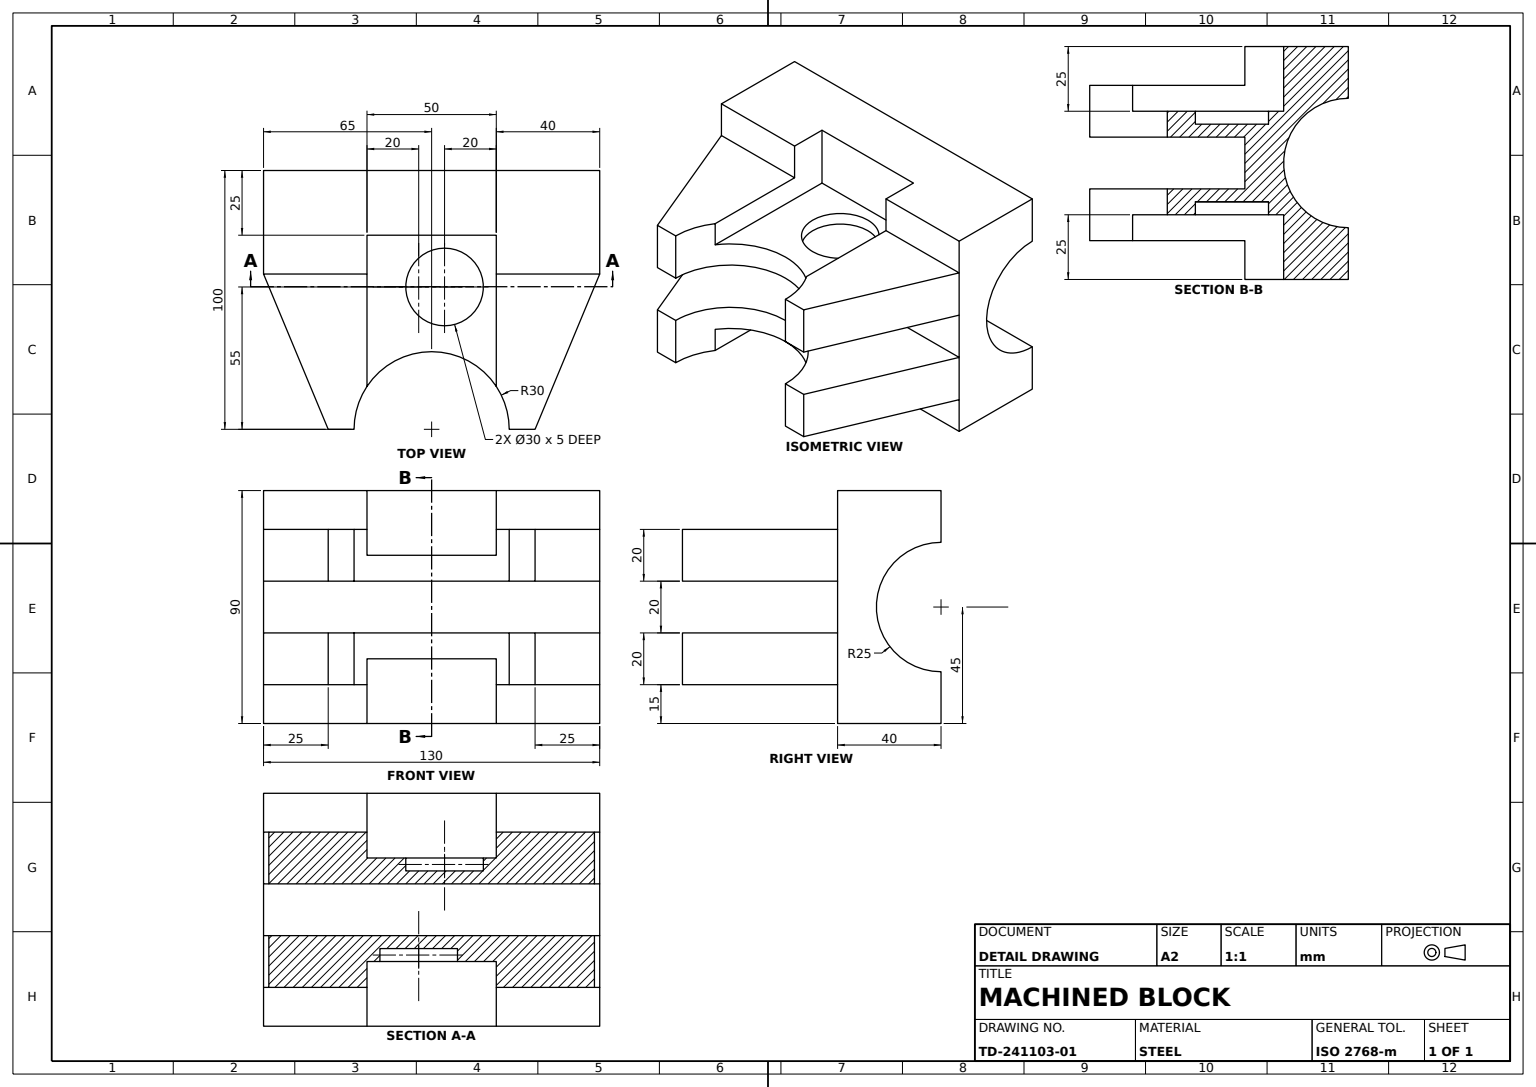
SolidWorks part; units mm, degrees
material "Plain Carbon Steel"
ref_plane "Front Plane" through (0, 0, 0) normal (0, 0, 1) x (1, 0, 0)
ref_plane "Top Plane" through (0, 0, 0) normal (0, 1, 0) x (1, 0, 0)
ref_plane "Right Plane" through (0, 0, 0) normal (1, 0, 0) x (0, 0, -1)
sketch "Base Block Sketch" plane through (0, 0, 0) normal (0, 0, 1) x (1, 0, 0)
  line L0 (0, 0) -> (130, 0)
  line L1 (130, 0) -> (130, 90)
  line L2 (130, 90) -> (0, 90)
  line L3 (0, 90) -> (0, 0)
  dimension "D1" = 130
  dimension "D2" = 90
extrude "Base Block 40" add sketch "Base Block Sketch" along normal blind 40
sketch "Side Pocket A Sketch" plane through (0, 0, 0) normal (0, -1, 0) x (1, 0, 0)
  line L0 (65, 40) -> (40, 40)
  line L1 (0, 40) -> (130, 40) construction
  line L2 (40, 40) -> (40, 25)
  line L3 (40, 25) -> (90, 25)
  line L4 (90, 25) -> (90, 40)
  line L5 (90, 40) -> (65, 40)
  line L6 (130, 40) -> (130, 0) construction
  line L7 (0, 0) -> (130, 0) construction
  dimension "D1" = 40
  dimension "D2" = 25
extrude "Side Pocket A 25" cut sketch "Side Pocket A Sketch" against normal blind 25
sketch "Side Pocket B Sketch" plane through (0, 90, 0) normal (0, 1, 0) x (1, 0, 0)
  line L0 (65, -40) -> (90, -40)
  line L1 (130, -40) -> (0, -40) construction
  line L2 (90, -40) -> (90, -25)
  line L3 (90, -25) -> (40, -25)
  line L4 (40, -25) -> (40, -40)
  line L5 (40, -40) -> (65, -40)
  line L6 (0, -40) -> (0, 0) construction
  line L7 (130, 0) -> (0, 0) construction
  dimension "D1" = 40
  dimension "D2" = 25
extrude "Side Pocket B 25" cut sketch "Side Pocket B Sketch" against normal blind 25
sketch "Upper Boss Sketch" plane through (0, 25, 0) normal (0, -1, 0) x (1, 0, 0)
  line L0 (40, 40) -> (40, 25) construction
  line L1 (90, 40) -> (40, 40) construction
  line L2 (65, 100) -> (105, 100)
  line L3 (105, 100) -> (130, 40)
  line L4 (130, 40) -> (0, 40)
  line L5 (65, 100) -> (25, 100)
  line L6 (25, 100) -> (0, 40)
  dimension "D1" = 65
  dimension "D2" = 60
extrude "Upper Boss 50" add sketch "Upper Boss Sketch" against normal blind 50
sketch "Web Boss Sketch" plane through (0, 25, 0) normal (0, -1, 0) x (1, 0, 0)
  line L0 (0, 40) -> (25, 100)
  line L1 (25, 100) -> (105, 100)
  line L2 (105, 100) -> (130, 40)
  line L3 (130, 40) -> (90, 40)
  line L4 (90, 40) -> (40, 40)
  line L5 (40, 40) -> (0, 40)
extrude "Web Boss 10" add sketch "Web Boss Sketch" along normal blind 10
sketch "Web Notch A Sketch" plane through (0, 15, 0) normal (0, -1, 0) x (1, 0, 0)
  line L0 (105, 100) -> (25, 100) construction
  line L1 (40, 100) -> (40, 40)
  line L2 (40, 40) -> (90, 40)
  line L3 (90, 40) -> (90, 100)
  line L4 (90, 100) -> (40, 100)
  arc A0 (40, 100) -> (90, 100) centre (65, 100) ccw
  line M2 (40, 40) -> (90, 40)
  line M5 (105, 100) -> (25, 100)
extrude "Web Notch A 10" cut sketch "Web Notch A Sketch" against normal blind 10 contours A0 M5 | A0 L1 L3 M2
sketch "Web Notch B Sketch" plane through (0, 75, 0) normal (0, 1, 0) x (1, 0, 0)
  line L0 (105, -100) -> (25, -100) construction
  line L1 (40, -100) -> (40, -40)
  line L2 (40, -40) -> (90, -40)
  line L3 (90, -40) -> (90, -100)
  line L4 (90, -100) -> (40, -100)
  arc A0 (90, -100) -> (40, -100) centre (65, -100) ccw
  line M1 (25, -100) -> (105, -100)
  line M4 (90, -40) -> (40, -40)
extrude "Web Notch B 10" cut sketch "Web Notch B Sketch" against normal blind 10 contours A0 L3 L1 M4 | A0 M1
sketch "Slot Cut A Sketch" plane through (0, 25, 0) normal (0, -1, 0) x (1, 0, 0)
  line L0 (90, 100) -> (40, 100) construction
  line L1 (35, 100) -> (95, 100)
  arc A0 (35, 100) -> (95, 100) centre (65, 100) ccw
  dimension "D1" = 30
extrude "Slot Cut A 60" cut sketch "Slot Cut A Sketch" against normal blind 60
sketch "Slot Cut B Sketch" plane through (0, 25, 0) normal (0, 1, 0) x (1, 0, 0)
  line L0 (40, -100) -> (40, -83.4169)
  line L1 (90, -100) -> (90, -83.4169)
  line L2 (90, -100) -> (95, -100)
  line L3 (40, -100) -> (35, -100)
  arc A0 (95, -100) -> (90, -83.4169) centre (65, -100) ccw
  arc A1 (40, -83.4169) -> (35, -100) centre (65, -100) ccw
extrude "Slot Cut B 60" cut sketch "Slot Cut B Sketch" against normal blind 60
sketch "Slot Cut C Sketch" plane through (0, 0, 100) normal (0, 0, 1) x (1, 0, 0)
  line L1 (105, 15) -> (95, 15) construction
  line L2 (25, 75) -> (25, 15) construction
  line L4 (25, 55) -> (105, 55)
  line L5 (105, 75) -> (105, 15) construction
  line L6 (105, 55) -> (130, 55)
  line L7 (0, 35) -> (0, 55)
  line L8 (130, 55) -> (130, 35)
  line L9 (130, 75) -> (130, 15) construction
  line L10 (130, 35) -> (0, 35)
  line L11 (0, 75) -> (0, 15) construction
  line L12 (0, 55) -> (25, 55)
  dimension "D1" = 20
  dimension "D2" = 40
extrude "Slot Cut C 60" cut sketch "Slot Cut C Sketch" against normal blind 60
sketch "Spot Face A Sketch" plane through (0, 25, 0) normal (0, -1, 0) x (1, 0, 0)
  line L0 (40, 83.4169) -> (40, 25) construction
  circle A0 centre (60, 45) radius 15
  dimension "D1" = 30
  dimension "D2" = 30
  dimension "D3" = 20
  dimension "D4" = 20
extrude "Spot Face A Ø30x5" cut sketch "Spot Face A Sketch" against normal blind 5
sketch "Spot Face B Sketch" plane through (0, 65, 0) normal (0, 1, 0) x (1, 0, 0)
  line L0 (90, -83.4169) -> (90, -25) construction
  circle A0 centre (70, -45) radius 15
  dimension "D1" = 30
  dimension "D2" = 30
  dimension "D3" = 20
  dimension "D4" = 20
extrude "Spot Face B Ø30x5" cut sketch "Spot Face B Sketch" against normal blind 5
sketch "Bearing Cradle Sketch" plane through (130, 0, 0) normal (1, 0, 0) x (0, 0, -1)
  line L0 (0, 0) -> (0, 90) construction
  line L1 (0, 70) -> (0, 20)
  arc A0 (0, 70) -> (0, 20) centre (0, 45) ccw
  dimension "D1" = 50
  dimension "D2" = 25
extrude "Bearing Cradle Ø50 Through" cut sketch "Bearing Cradle Sketch" against normal blind 130
